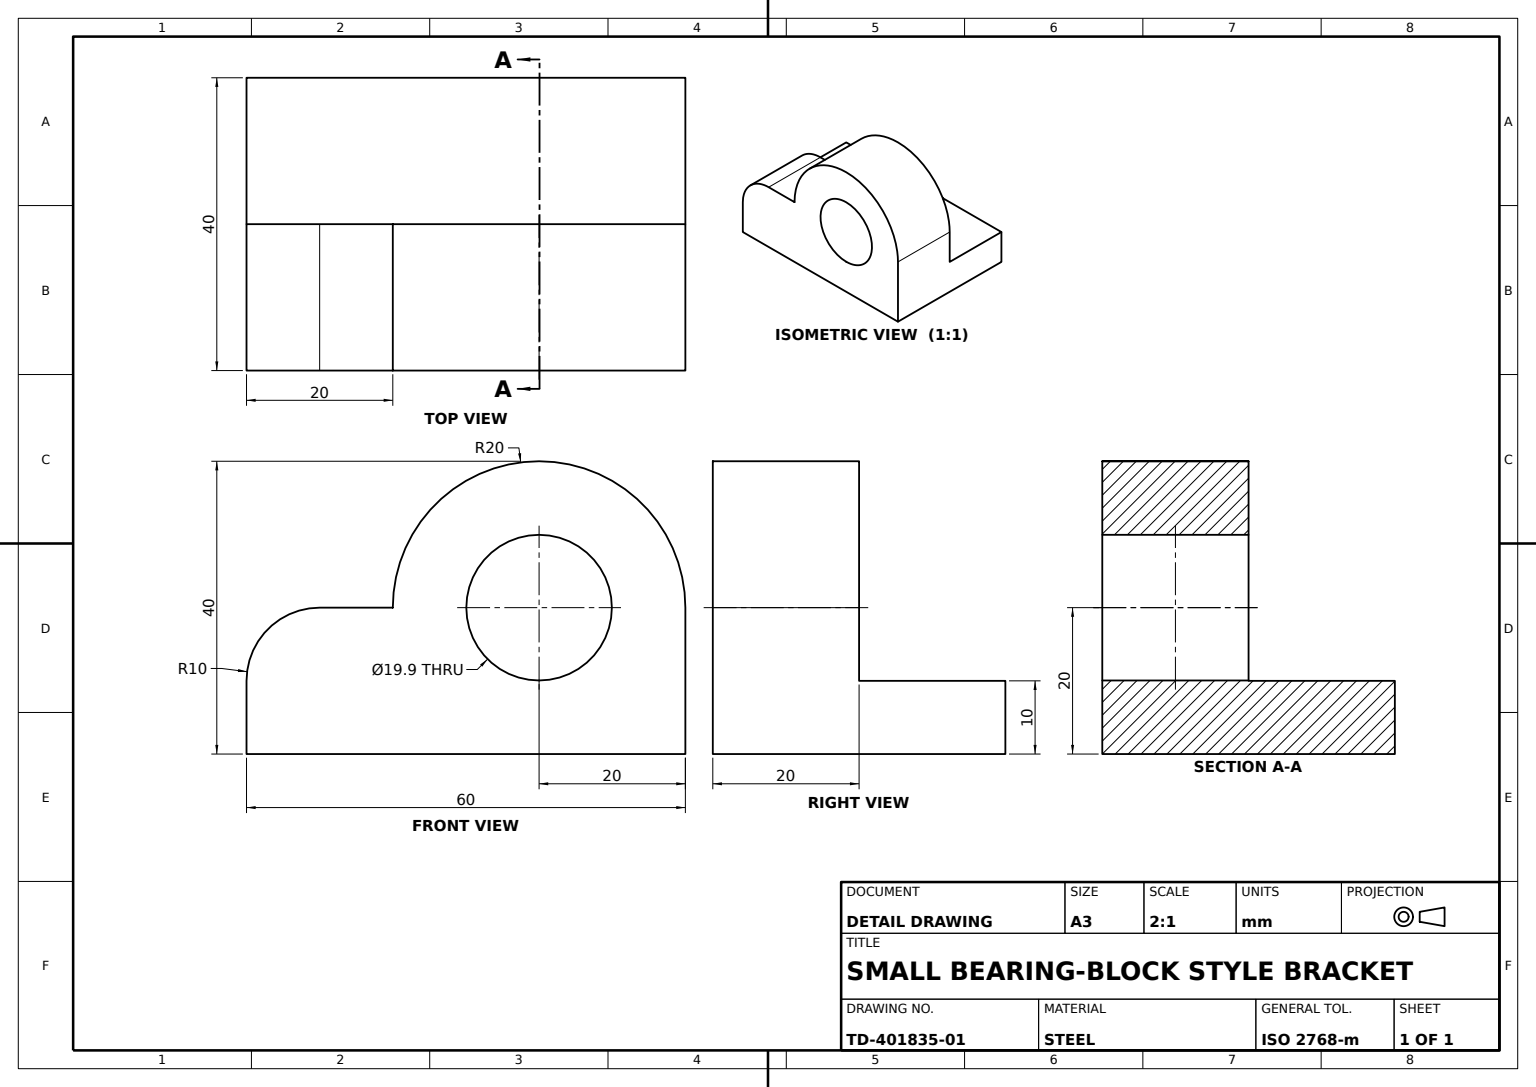
SolidWorks part; units mm, degrees
material "Plain Carbon Steel"
ref_plane "Front Plane" through (0, 0, 0) normal (0, 0, 1) x (1, 0, 0)
ref_plane "Top Plane" through (0, 0, 0) normal (0, 1, 0) x (1, 0, 0)
ref_plane "Right Plane" through (0, 0, 0) normal (1, 0, 0) x (0, 0, -1)
sketch "Bracket Profile Sketch" plane through (0, 0, 0) normal (1, 0, 0) x (0, 0, -1)
  line L0 (0, 0) -> (40, 0)
  line L1 (40, 0) -> (40, 10)
  line L5 (0, 40) -> (0, 0)
  line L6 (40, 10) -> (20, 10)
  line L7 (20, 10) -> (20, 40)
  line L8 (20, 40) -> (0, 40)
  dimension "D1" = 20
  dimension "D2" = 20
  dimension "D3" = 10
  dimension "D4" = 40
extrude "Bracket Body" add sketch "Bracket Profile Sketch" along normal mid plane 60
sketch "Boss Rounding Sketch" plane through (0, 0, -20) normal (0, 0, -1) x (-1, 0, 0)
  line L0 (-30, 0) -> (-30, 20) construction
  line L1 (-30, 10) -> (-30, 40) construction
  line L2 (-30, 20) -> (-10, 20) construction
  line L3 (30, 10) -> (30, 40) construction
  circle A1 centre (-10, 20) radius 9.95
  dimension "D1" = 19.9
  dimension "D2" = 40
extrude "Boss Rounding Cut" cut sketch "Boss Rounding Sketch" against normal blind 60
sketch "Bore Sketch" plane through (0, 0, -20) normal (0, 0, -1) x (-1, 0, 0)
  line L0 (10, 20) -> (20, 20)
  line L2 (30, 10) -> (-30, 10)
  line L3 (-30, 10) -> (-30, 20)
  line L4 (-30, 20) -> (-30, 40)
  line L5 (-30, 40) -> (30, 40)
  line L6 (30, 40) -> (30, 10)
  arc A0 (10, 20) -> (-30, 20) centre (-10, 20) ccw
  arc A2 (30, 10) -> (20, 20) centre (20, 10) ccw
  line M8 (30, 10) -> (30, 40)
  line M9 (30, 40) -> (-30, 40)
  line M10 (-30, 40) -> (-30, 10)
  dimension "D1" = 10
extrude "Bore Cut" cut sketch "Bore Sketch" against normal blind 60 contours A0 L5 M10 | A2 A0 L0 M8 M9
